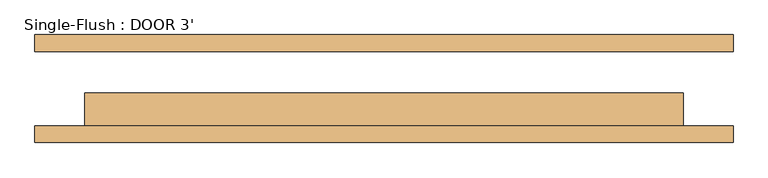
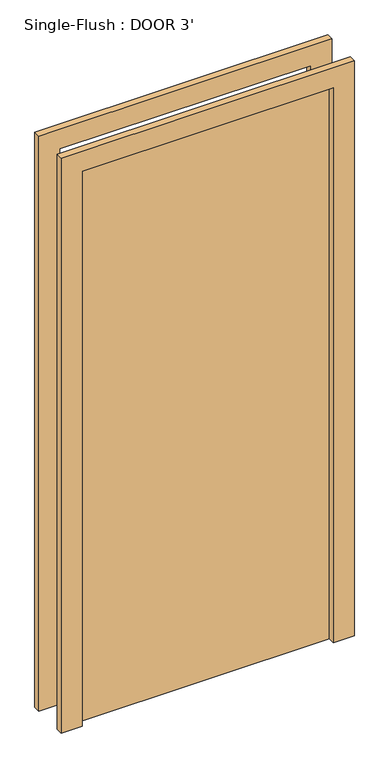
"""IFC4 building model written with IfcOpenShell, lengths in millimetres: door geometry, Single-Flush : DOOR 3'."""

from ifc_helpers import new_model, si_unit, frame, origin, origin_with_axes, place, context, project, spatial, polyline, outline, extrude, source, transform, mapped, element, save


def single_flush_door_3_305aa2a5(model_context):
    return source(origin(), model_context, "Body", "SweptSolid", [
        extrude(outline(polyline([(2209.8, -533.4), (0.0, -533.4), (0.0, -457.2), (2133.6, -457.2), (2133.6, 457.2), (0.0, 457.2), (0.0, 533.4), (2209.8, 533.4), (2209.8, -533.4)])), frame((0.0, -82.55, 0.0), z_axis=(0.0, 1.0, 0.0), x_axis=(0.0, 0.0, 1.0)), (0.0, 0.0, 1.0), 25.4),
        extrude(outline(polyline([(2209.8, 533.4), (2209.8, -533.4), (0.0, -533.4), (0.0, -457.2), (2133.6, -457.2), (2133.6, 457.2), (0.0, 457.2), (0.0, 533.4), (2209.8, 533.4)])), frame((0.0, 57.15, 0.0), z_axis=(0.0, 1.0, 0.0), x_axis=(0.0, 0.0, 1.0)), (0.0, 0.0, 1.0), 25.4),
        extrude(outline(polyline([(457.2, -6.35), (457.2, -57.15), (-457.2, -57.15), (-457.2, -6.35), (457.2, -6.35)])), origin_with_axes(), (0.0, 0.0, 1.0), 2133.6),
    ])


if __name__ == "__main__":
    model = new_model("IFC4")
    model_context = context("Model", 3, world=origin())
    ifc_project = project(units=[si_unit("LENGTHUNIT", "METRE", prefix="MILLI")], contexts=[model_context])
    site = spatial("IfcSite", under=ifc_project)
    building = spatial("IfcBuilding", under=site)
    placement = place(None, origin())
    single_flush_door_3_shape = single_flush_door_3_305aa2a5(model_context)
    element("IfcDoor", 1, ObjectType="Single-Flush : DOOR 3'", at=placement, inside=building, context=model_context, shape_type="MappedRepresentation", body=[
        mapped(single_flush_door_3_shape, transform((0.0, 0.0, 0.0), x_axis=(1.0, 0.0, 0.0), y_axis=(0.0, 1.0, 0.0), z_axis=(0.0, 0.0, 1.0))),
    ])
    save(model, "model.ifc")

# Revit data of these elements
# Type "Single-Flush : DOOR 3'"
#   Type Mark = "9"
#   Construction Type Id = "MDOOR"
#   Assembly Code = "C1020"
#   Analytic Construction = "Metal"
#   Thickness = 0' - 2"
#   Heat Transfer Coefficient (U) = 0.651978 BTU/(h·ft²·°F)
#   Height = 7' - 0"
#   Trim Projection Ext = 0' - 1"
#   Trim Projection Int = 0' - 1"
#   Trim Width = 0' - 3"
#   Width = 3' - 0"
#   Define Thermal Properties by = 1
#   Door Material = Door - Panel
#   Frame Material = Door - Frame
#   Visual Light Transmittance = 0
#   Solar Heat Gain Coefficient = 0
#   Function = (empty or 0)
#   Wall Closure = (empty or 0)
# Element 1 (IfcDoor, "Single-Flush : DOOR 3'")
#   Materials on its faces: "Door - Frame", "Door - Panel"
# Materials
#   "Door - Panel": class "Wood", colour RGB 210 159 95, transparency 0, Cost = 0
#   "Door - Frame": colour RGB 118 70 51, transparency 0, Cost = 0
